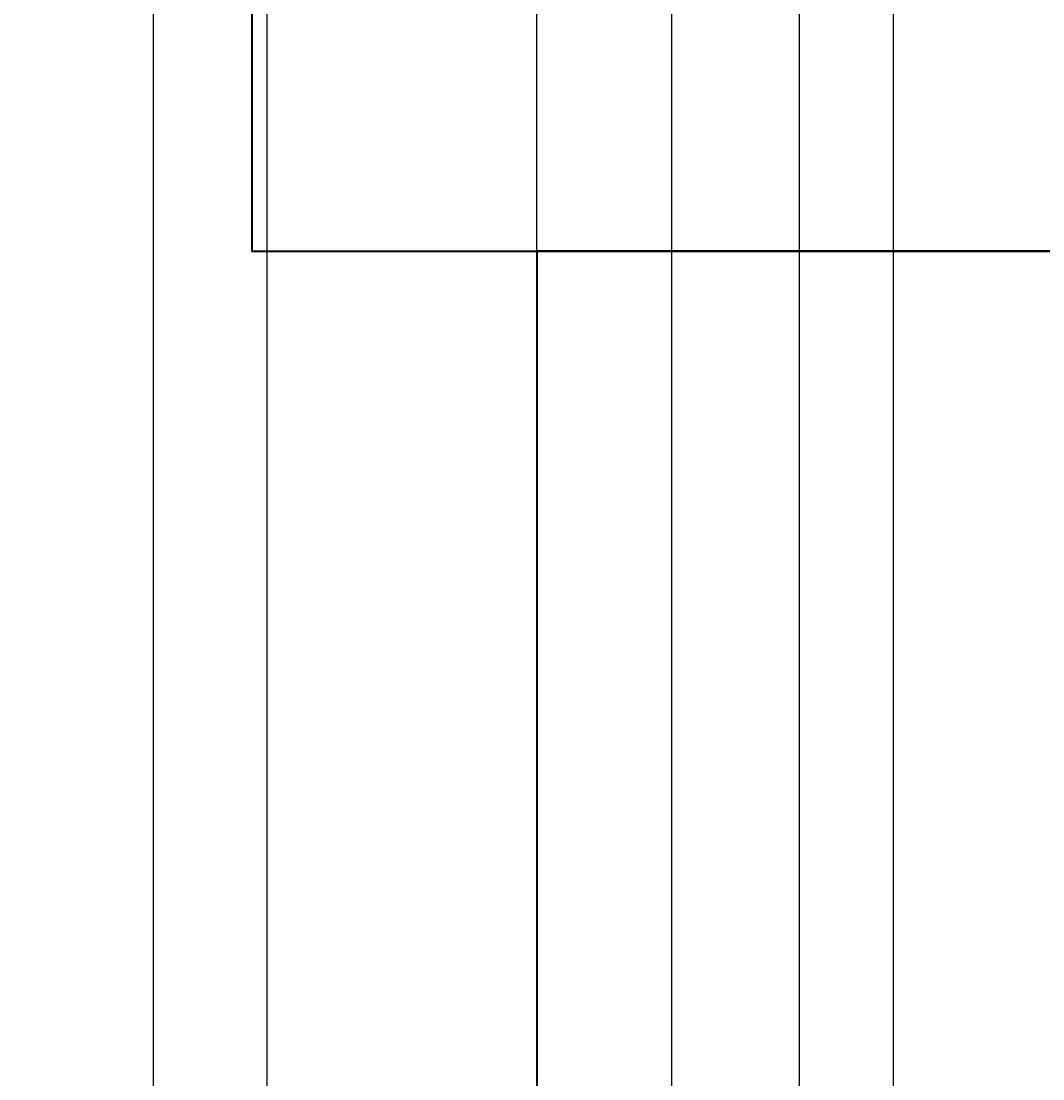
# Model space of a CAD drawing. Units: inches. Extents: x -6 to 289, y -8 to 323.
# Tile 77 of 107: x 104 to 126, y 229 to 252. Entities that reach past the tile are written whole.
import ezdxf

# ---------------------------------------------------------------- set-up
doc = ezdxf.new("R2010")
doc.units = ezdxf.units.IN
doc.header["$MEASUREMENT"] = 0
doc.layers.add('A-ANNO-DIMS', color=2, linetype='Continuous', lineweight=18)
doc.layers.add('A-ELEV', color=7, linetype='Continuous', lineweight=35)
doc.styles.get("Standard").update_dxf_attribs({"font": 'arial.ttf'})
doc.dimstyles.get("Standard").update_dxf_attribs({"dimtxt": 0.18, "dimasz": 0.18, "dimexe": 0.18, "dimexo": 0.0625, "dimgap": 0.09, "dimtad": 0, "dimtih": 1, "dimtoh": 1, "dimdec": 4, "dimzin": 0, "dimdsep": 46, "dimtxsty": 'Standard', "dimcen": 0.09, "dimadec": 0, "dimazin": 0, "dimtfac": 1, "dimtdec": 4, "dimtofl": 0, "dimtmove": 0, "dimatfit": 3, "dimfxl": 1, "dimtolj": 1, "dimtzin": 0, "dimarcsym": 0})

# ---------------------------------------------------------------- blocks, each defined once
blk = doc.blocks.new('*D10')
at = {"layer": 'A-ANNO-DIMS', "color": 0, "lineweight": -2, "transparency": 16777216}
for p, q in [((115.164, 307.351), (115.164, 322.969)), ((126.883, 226.717), (126.883, 322.969)), ((115.344, 322.789), (120.639, 322.789)), ((126.703, 322.789), (121.408, 322.789))]:
    blk.add_line(p, q, dxfattribs=at)
at = {"layer": 'A-ANNO-DIMS', "color": 0, "transparency": 16777216}
for points in [[(115.344, 322.819), (115.344, 322.759), (115.164, 322.789)], [(126.703, 322.819), (126.703, 322.759), (126.883, 322.789)]]:
    blk.add_solid(points, dxfattribs=at)
at = {"layer": 'Defpoints', "color": 0, "transparency": 16777216}
for p in [(126.883, 322.789), (115.164, 307.289), (126.883, 226.654)]:
    blk.add_point(p, dxfattribs=at)
at = {"layer": 'A-ANNO-DIMS', "color": 0, "transparency": 16777216, "insert": (121.024, 322.789), "char_height": 0.18, "attachment_point": 5}
blk.add_mtext('\\A1;11.72', dxfattribs=at)
blk = doc.blocks.new('*D27')
at = {"layer": 'A-ANNO-DIMS', "color": 0, "lineweight": -2, "transparency": 16777216}
for p, q in [((19.226, 307.289), (288.653, 307.289)), ((288.473, 307.109), (288.473, 277.471)), ((288.473, 247.469), (288.473, 277.107)), ((247.226, 247.289), (288.653, 247.289))]:
    blk.add_line(p, q, dxfattribs=at)
at = {"layer": 'A-ANNO-DIMS', "color": 0, "transparency": 16777216}
for points in [[(288.443, 307.109), (288.503, 307.109), (288.473, 307.289)], [(288.443, 247.469), (288.503, 247.469), (288.473, 247.289)]]:
    blk.add_solid(points, dxfattribs=at)
at = {"layer": 'Defpoints', "color": 0, "transparency": 16777216}
for p in [(19.164, 307.289), (288.473, 307.289), (247.164, 247.289)]:
    blk.add_point(p, dxfattribs=at)
at = {"layer": 'A-ANNO-DIMS', "color": 0, "transparency": 16777216, "insert": (288.473, 277.289), "char_height": 0.18, "attachment_point": 5}
blk.add_mtext('\\A1;60', dxfattribs=at)
blk = doc.blocks.new('*D58')
at = {"layer": 'A-ANNO-DIMS', "color": 0, "lineweight": -2, "transparency": 16777216}
for p, q in [((106.634, 68.495), (106.634, 322.969)), ((123.094, 68.495), (123.094, 322.969)), ((106.814, 322.789), (114.479, 322.789)), ((122.914, 322.789), (115.249, 322.789))]:
    blk.add_line(p, q, dxfattribs=at)
at = {"layer": 'A-ANNO-DIMS', "color": 0, "transparency": 16777216}
for points in [[(106.814, 322.819), (106.814, 322.759), (106.634, 322.789)], [(122.914, 322.819), (122.914, 322.759), (123.094, 322.789)]]:
    blk.add_solid(points, dxfattribs=at)
at = {"layer": 'Defpoints', "color": 0, "transparency": 16777216}
for p in [(123.094, 322.789), (106.634, 68.432), (123.094, 68.432)]:
    blk.add_point(p, dxfattribs=at)
at = {"layer": 'A-ANNO-DIMS', "color": 0, "transparency": 16777216, "insert": (114.864, 322.789), "char_height": 0.18, "attachment_point": 5}
blk.add_mtext('\\A1;16.46', dxfattribs=at)
blk = doc.blocks.new('*D73')
at = {"layer": 'A-ANNO-DIMS', "color": 0, "lineweight": -2, "transparency": 16777216}
for p, q in [((121.008, 51.148), (121.008, 322.969)), ((135.296, 51.148), (135.296, 322.969)), ((121.188, 322.789), (127.697, 322.789)), ((135.116, 322.789), (128.607, 322.789))]:
    blk.add_line(p, q, dxfattribs=at)
at = {"layer": 'A-ANNO-DIMS', "color": 0, "transparency": 16777216}
for points in [[(121.188, 322.819), (121.188, 322.759), (121.008, 322.789)], [(135.116, 322.819), (135.116, 322.759), (135.296, 322.789)]]:
    blk.add_solid(points, dxfattribs=at)
at = {"layer": 'Defpoints', "color": 0, "transparency": 16777216}
for p in [(135.296, 322.789), (121.008, 51.085), (135.296, 51.085)]:
    blk.add_point(p, dxfattribs=at)
at = {"layer": 'A-ANNO-DIMS', "color": 0, "transparency": 16777216, "insert": (128.152, 322.789), "char_height": 0.18, "attachment_point": 5}
blk.add_mtext('\\A1;14.288', dxfattribs=at)
blk = doc.blocks.new('*D92')
at = {"layer": 'A-ANNO-DIMS', "color": 0, "lineweight": -2, "transparency": 16777216}
for p, q in [((109.164, 127.351), (109.164, 322.969)), ((115.164, 162.411), (115.164, 322.969)), ((109.344, 322.789), (112.014, 322.789)), ((114.984, 322.789), (112.313, 322.789))]:
    blk.add_line(p, q, dxfattribs=at)
at = {"layer": 'A-ANNO-DIMS', "color": 0, "transparency": 16777216}
for points in [[(109.344, 322.819), (109.344, 322.759), (109.164, 322.789)], [(114.984, 322.819), (114.984, 322.759), (115.164, 322.789)]]:
    blk.add_solid(points, dxfattribs=at)
at = {"layer": 'Defpoints', "color": 0, "transparency": 16777216}
for p in [(115.164, 322.789), (115.164, 162.348), (109.164, 127.289)]:
    blk.add_point(p, dxfattribs=at)
at = {"layer": 'A-ANNO-DIMS', "color": 0, "transparency": 16777216, "insert": (112.164, 322.789), "char_height": 0.18, "attachment_point": 5}
blk.add_mtext('\\A1;6', dxfattribs=at)
blk = doc.blocks.new('*D93')
at = {"layer": 'A-ANNO-DIMS', "color": 0, "lineweight": -2, "transparency": 16777216}
for p, q in [((115.164, 162.411), (115.164, 322.969)), ((118.164, 159.411), (118.164, 322.969)), ((115.344, 322.789), (116.515, 322.789)), ((117.984, 322.789), (116.813, 322.789))]:
    blk.add_line(p, q, dxfattribs=at)
at = {"layer": 'A-ANNO-DIMS', "color": 0, "transparency": 16777216}
for points in [[(115.344, 322.819), (115.344, 322.759), (115.164, 322.789)], [(117.984, 322.819), (117.984, 322.759), (118.164, 322.789)]]:
    blk.add_solid(points, dxfattribs=at)
at = {"layer": 'Defpoints', "color": 0, "transparency": 16777216}
for p in [(118.164, 322.789), (115.164, 162.348), (118.164, 159.348)]:
    blk.add_point(p, dxfattribs=at)
at = {"layer": 'A-ANNO-DIMS', "color": 0, "transparency": 16777216, "insert": (116.664, 322.789), "char_height": 0.18, "attachment_point": 5}
blk.add_mtext('\\A1;3', dxfattribs=at)
blk = doc.blocks.new('*D94')
at = {"layer": 'A-ANNO-DIMS', "color": 0, "lineweight": -2, "transparency": 16777216}
for p, q in [((118.164, 159.411), (118.164, 322.969)), ((161.552, 159.411), (161.552, 322.969)), ((118.344, 322.789), (139.46, 322.789)), ((161.372, 322.789), (140.256, 322.789))]:
    blk.add_line(p, q, dxfattribs=at)
at = {"layer": 'A-ANNO-DIMS', "color": 0, "transparency": 16777216}
for points in [[(118.344, 322.819), (118.344, 322.759), (118.164, 322.789)], [(161.372, 322.819), (161.372, 322.759), (161.552, 322.789)]]:
    blk.add_solid(points, dxfattribs=at)
at = {"layer": 'Defpoints', "color": 0, "transparency": 16777216}
for p in [(161.552, 322.789), (118.164, 159.348), (161.552, 159.348)]:
    blk.add_point(p, dxfattribs=at)
at = {"layer": 'A-ANNO-DIMS', "color": 0, "transparency": 16777216, "insert": (139.858, 322.789), "char_height": 0.18, "attachment_point": 5}
blk.add_mtext('\\A1;43.39', dxfattribs=at)

msp = doc.modelspace()

# ---------------------------------------------------------------- linework, layer by layer
at = {"layer": 'A-ELEV'}
for p, q in [((247.1638, 247.2888), (115.1638, 247.2888)), ((115.1638, 247.2888), (247.1638, 247.2888)), ((115.1638, 247.2888), (115.1638, 139.2888))]:
    msp.add_line(p, q, dxfattribs=at)
msp.add_lwpolyline([(115.1638, 259.2888), (108.8227, 259.2888), (108.8227, 247.2888), (115.1638, 247.2888)], dxfattribs=at)

# ---------------------------------------------------------------- dimensions: what is measured, and where the dimension line sits
at = {"layer": 'A-ANNO-DIMS'}
for base, p1, p2, override, picture, middle in [((123.094, 322.7888), (106.634, 68.4322), (123.094, 68.4322), {"dimdec": 2, "dimlfac": 1, "dimrnd": 0, "dimzin": 0, "dimdsep": 46, "dimlunit": 2}, '*D58', (114.864, 322.7888)), ((115.1638, 322.7888), (109.1638, 127.2888), (115.1638, 162.3484), {"dimdec": 0, "dimlfac": 1, "dimrnd": 0, "dimzin": 0, "dimdsep": 46, "dimlunit": 2}, '*D92', (112.1638, 322.7888)), ((126.8835, 322.7888), (115.1638, 307.2888), (126.8835, 226.654), {"dimdec": 2, "dimlfac": 1, "dimrnd": 0, "dimzin": 0, "dimdsep": 46, "dimlunit": 2}, '*D10', (121.0236, 322.7888)), ((118.1638, 322.7888), (115.1638, 162.3484), (118.1638, 159.3484), {"dimdec": 0, "dimlfac": 1, "dimrnd": 0, "dimzin": 0, "dimdsep": 46, "dimlunit": 2}, '*D93', (116.6638, 322.7888)), ((161.5522, 322.7888), (118.1638, 159.3484), (161.5522, 159.3484), {"dimdec": 2, "dimlfac": 1, "dimrnd": 0, "dimzin": 0, "dimdsep": 46, "dimlunit": 2}, '*D94', (139.858, 322.7888)), ((135.296, 322.7888), (121.008, 51.0851), (135.296, 51.0851), {"dimdec": 3, "dimlfac": 1, "dimrnd": 0, "dimzin": 0, "dimdsep": 46, "dimlunit": 2}, '*D73', (128.152, 322.7888))]:
    dim = msp.add_linear_dim(base=base, p1=p1, p2=p2, dimstyle='Standard', override=override, dxfattribs=at)
    dim.commit()
    dim.dimension.update_dxf_attribs({"geometry": picture, "text_midpoint": middle})
dim = msp.add_linear_dim(base=(288.4733, 307.2888), p1=(247.1638, 247.2888), p2=(19.1638, 307.2888), angle=90, dimstyle='Standard', override={"dimdec": 0, "dimlfac": 1, "dimrnd": 0, "dimzin": 0, "dimdsep": 46, "dimlunit": 2}, dxfattribs=at)
dim.commit()
dim.dimension.update_dxf_attribs({"geometry": '*D27', "text_midpoint": (288.4733, 277.2888)})

doc.saveas('drawing.dxf')
